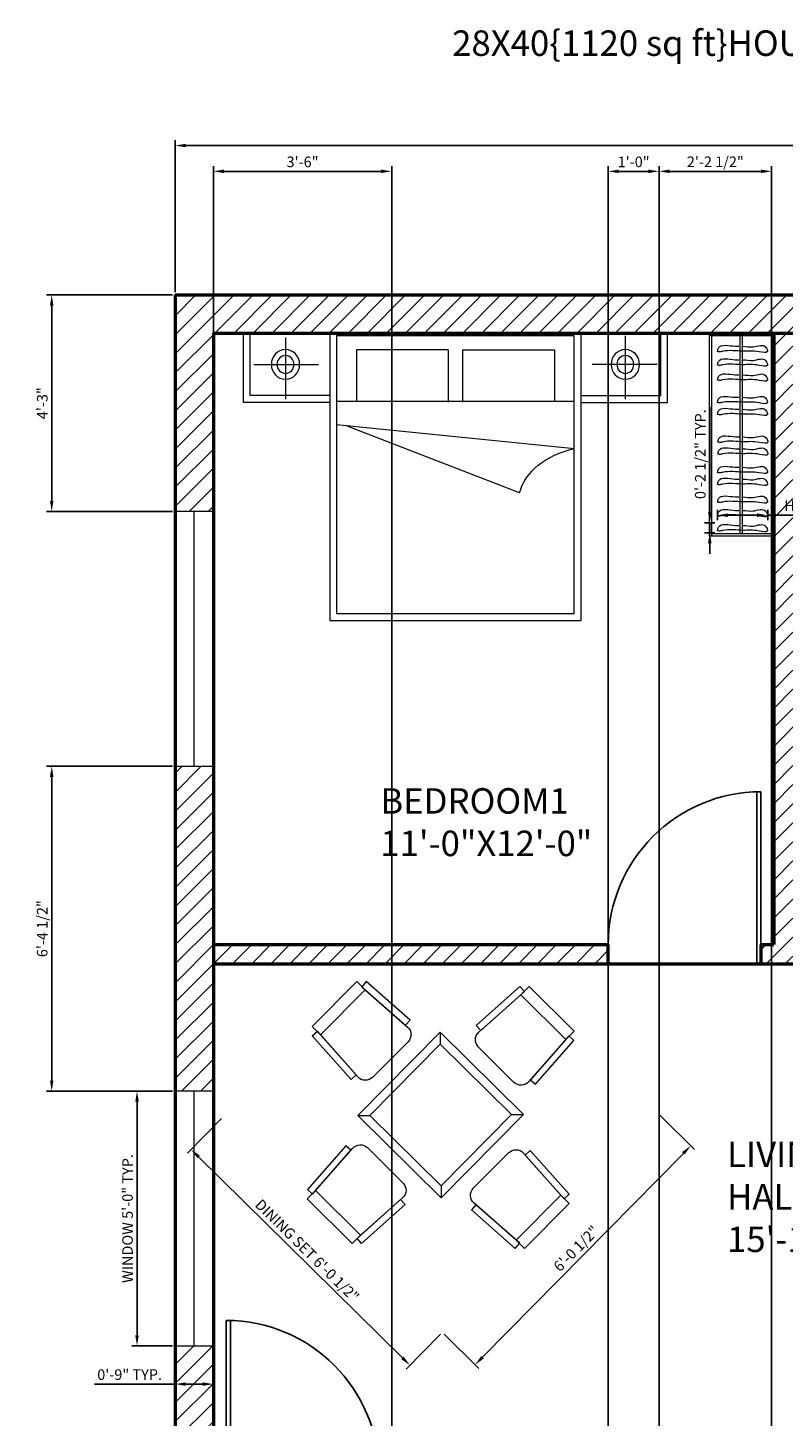
# Model space of a CAD drawing. Units: inches. Extents: x 3887 to 4286, y 884 to 1458.
# Tile 3 of 4: x 3887 to 4065, y 1131 to 1458. Entities that reach past the tile are written whole.
import ezdxf

# ---------------------------------------------------------------- set-up
doc = ezdxf.new("R2010")
doc.units = ezdxf.units.IN
for name, color, linetype, lineweight in [('A-ANNO-DIMS', 2, 'Continuous', 18), ('A-ANNO-TEXT', 7, 'Continuous', 25), ('A-AREA-IDEN', 7, 'Continuous', 25), ('A-DOOR', 3, 'Continuous', 25), ('A-FURN', 8, 'Continuous', 18), ('A-GLAZ', 4, 'Continuous', 18), ('A-WALL', 7, 'Continuous', 50), ('A-WALL-PATT', 252, 'Continuous', 13)]:
    doc.layers.add(name, color=color, linetype=linetype, lineweight=lineweight)
doc.styles.get("Standard").update_dxf_attribs({"font": 'arial.ttf'})
doc.dimstyles.new('ISO-25', dxfattribs={"dimtxt": 2.5, "dimasz": 2.5, "dimexe": 1.25, "dimexo": 0.625, "dimtad": 1, "dimdec": 0, "dimlunit": 3, "dimtxsty": 'Standard', "dimcen": 2.5, "dimadec": 0, "dimazin": 0, "dimtfac": 1, "dimtdec": 0, "dimtmove": 0, "dimatfit": 3, "dimfxl": 1, "dimarcsym": 0})

# ---------------------------------------------------------------- blocks, each defined once
blk = doc.blocks.new('4 Person Square 01')
for p, q in [((618.5, 273.1), (568.5, 323.1)), ((1268.5, 323.1), (1218.5, 273.1)), ((618.5, -326.9), (568.5, -376.9)), ((1268.5, -376.9), (1218.5, -326.9))]:
    blk.add_line(p, q)
for points in [[(734, 501.7), (693.7, 504.3), (716.8, 852.8), (757.1, 850.2)], [(755.6, 821.7), (755.9, 892.5), (1135, 890.7), (1134.7, 819.9)], [(1153.2, 499.8), (1193.6, 502), (1173.7, 850.7), (1133.4, 848.5)], [(568.5, 323.1), (1268.5, 323.1), (1268.5, -376.9), (568.5, -376.9)], [(618.5, 273.1), (1218.5, 273.1), (1218.5, -326.9), (618.5, -326.9)], [(69.9, -189.9), (-0.9, -189.6), (0.9, 189.6), (71.7, 189.3)], [(391.8, 207.8), (389.6, 248.1), (40.9, 228.3), (43.1, 188)], [(1447.2, 157.6), (1449.8, 197.9), (1798.3, 174.8), (1795.7, 134.5)], [(1767.1, 136), (1837.9, 135.7), (1836.1, -243.4), (1765.4, -243.1)], [(389.9, -211.4), (387.3, -251.7), (38.8, -228.6), (41.4, -188.3)], [(1445.2, -261.6), (1447.4, -302), (1796.1, -282.1), (1793.9, -241.8)], [(683.8, -553.6), (643.5, -555.8), (663.3, -904.5), (703.6, -902.3)], [(1103, -555.6), (1143.3, -558.2), (1120.2, -906.7), (1079.9, -904.1)], [(1081.5, -875.5), (1081.2, -946.3), (702, -944.5), (702.3, -873.8)]]:
    blk.add_lwpolyline(points, close=True)
for points in [[(1154, 483.4, -0.431982), (1093.8, 420.1), (792.7, 421.5, -0.431982), (733.1, 485.4), (755.6, 821.7), (1134.7, 819.9)], [(408.2, 208.6, -0.431982), (471.5, 148.4), (470.1, -152.7, -0.431982), (406.2, -212.3), (69.9, -189.9), (71.7, 189.3)], [(1428.9, -262.4, -0.431982), (1365.5, -202.2), (1367, 98.9, -0.431982), (1430.9, 158.5), (1767.1, 136), (1765.4, -243.1)], [(683, -537.3, -0.431982), (743.2, -473.9), (1044.3, -475.4, -0.431982), (1103.9, -539.3), (1081.5, -875.5), (702.3, -873.8)]]:
    blk.add_lwpolyline(points, format="xyb", close=True)
blk = doc.blocks.new('*D10')
at = {"layer": 'A-ANNO-DIMS', "color": 0, "lineweight": -2, "transparency": 16777216}
for p, q in [((3922.18, 1395.27), (3922.18, 1431.07)), ((3924.68, 1429.82), (4252.68, 1429.82)), ((4255.18, 1395.27), (4255.18, 1431.07))]:
    blk.add_line(p, q, dxfattribs=at)
at = {"layer": 'A-ANNO-DIMS', "color": 0, "transparency": 16777216}
for points in [[(3924.68, 1430.23), (3924.68, 1429.4), (3922.18, 1429.82)], [(4252.68, 1430.23), (4252.68, 1429.4), (4255.18, 1429.82)]]:
    blk.add_solid(points, dxfattribs=at)
at = {"layer": 'Defpoints', "color": 0, "transparency": 16777216}
for p in [(4255.18, 1429.82), (3922.18, 1394.64), (4255.18, 1394.64)]:
    blk.add_point(p, dxfattribs=at)
at = {"layer": 'A-ANNO-DIMS', "color": 0, "transparency": 16777216, "insert": (4088.68, 1431.72), "char_height": 2.5, "attachment_point": 5}
blk.add_mtext('27\'-9"', dxfattribs=at)
blk = doc.blocks.new('DOOR-SWING-36IN')
for p, q in [((35, 0), (35, 40.5)), ((36, 4.5), (36, 40.5))]:
    blk.add_line(p, q)
blk.add_arc((36, 4.5), 36, 90, 180)
blk = doc.blocks.new('WIN-GLAZ-60IN')
for p, q in [((60, 9), (0, 9)), ((0, 4.5), (60, 4.5)), ((0, 0), (60, 0))]:
    blk.add_line(p, q)
blk = doc.blocks.new('CLOSET-HANGER')
for points, knots in [([(5.84, 1.53), (5.89, 1.53), (6.71, 1.5), (8.51, 1.02), (11.18, 2.34), (12.19, -0.34), (8.75, 0.58), (5.91, 0.14), (2.52, 0.71), (0.53, 0.12), (0.14, 0.25), (0, 0.3)], [256.949798, 256.949798, 256.949798, 256.949798, 263.372126, 359.428036, 478.655159, 522.640662, 597.66786, 752.004169, 941.88133, 973.527729, 990.309099, 990.309099, 990.309099, 990.309099]), ([(0.03, 0.25), (0.09, 0.56), (0.4, 2.27), (3.16, 1.49), (4.81, 1.52), (5.08, 1.53)], [0, 0, 0, 0, 35.911014, 192.421107, 225.897258, 225.897258, 225.897258, 225.897258])]:
    blk.add_open_spline(points, degree=3, knots=knots)
blk = doc.blocks.new('*D15')
at = {"layer": 'A-ANNO-DIMS', "color": 0, "lineweight": -2, "transparency": 16777216}
for p, q in [((4049.91, 1341.61), (4049.91, 1344.01)), ((4061.79, 1341.61), (4061.79, 1344.01)), ((4052.41, 1342.76), (4059.29, 1342.76)), ((4061.79, 1342.76), (4096.55, 1342.76))]:
    blk.add_line(p, q, dxfattribs=at)
at = {"layer": 'A-ANNO-DIMS', "color": 0, "transparency": 16777216}
for points in [[(4052.41, 1343.18), (4052.41, 1342.35), (4049.91, 1342.76)], [(4059.29, 1343.18), (4059.29, 1342.35), (4061.79, 1342.76)]]:
    blk.add_solid(points, dxfattribs=at)
at = {"layer": 'Defpoints', "color": 0, "transparency": 16777216}
for p in [(4049.91, 1340.98), (4061.79, 1342.76), (4061.79, 1340.98)]:
    blk.add_point(p, dxfattribs=at)
at = {"layer": 'A-ANNO-DIMS', "color": 0, "transparency": 16777216, "insert": (4080.42, 1344.68), "char_height": 2.5, "attachment_point": 5}
blk.add_mtext('HANGER 1\'-0" TYP.', dxfattribs=at)
blk = doc.blocks.new('*D16')
at = {"layer": 'A-ANNO-DIMS', "color": 0, "lineweight": -2, "transparency": 16777216}
for p, q in [((4048.13, 1343.48), (4048.13, 1368.3)), ((4049.29, 1340.98), (4046.88, 1340.98)), ((4048.13, 1338.64), (4048.13, 1340.98)), ((4049.29, 1338.64), (4046.88, 1338.64)), ((4048.13, 1336.14), (4048.13, 1333.64))]:
    blk.add_line(p, q, dxfattribs=at)
at = {"layer": 'A-ANNO-DIMS', "color": 0, "transparency": 16777216}
for points in [[(4047.71, 1343.48), (4048.55, 1343.48), (4048.13, 1340.98)], [(4047.71, 1336.14), (4048.55, 1336.14), (4048.13, 1338.64)]]:
    blk.add_solid(points, dxfattribs=at)
at = {"layer": 'Defpoints', "color": 0, "transparency": 16777216}
for p in [(4048.13, 1340.98), (4049.91, 1340.98), (4049.91, 1338.64)]:
    blk.add_point(p, dxfattribs=at)
at = {"layer": 'A-ANNO-DIMS', "color": 0, "transparency": 16777216, "insert": (4046.21, 1357.14), "char_height": 2.5, "attachment_point": 5, "rotation": 90}
blk.add_mtext('0\'-2 1/2" TYP.', dxfattribs=at)
blk = doc.blocks.new('*D17')
at = {"layer": 'A-ANNO-DIMS', "color": 0, "lineweight": -2, "transparency": 16777216}
for p, q in [((3921.56, 1207.14), (3911.93, 1207.14)), ((3913.18, 1149.64), (3913.18, 1204.64)), ((3921.56, 1147.14), (3911.93, 1147.14))]:
    blk.add_line(p, q, dxfattribs=at)
at = {"layer": 'A-ANNO-DIMS', "color": 0, "transparency": 16777216}
for points in [[(3912.77, 1204.64), (3913.6, 1204.64), (3913.18, 1207.14)], [(3912.77, 1149.64), (3913.6, 1149.64), (3913.18, 1147.14)]]:
    blk.add_solid(points, dxfattribs=at)
at = {"layer": 'Defpoints', "color": 0, "transparency": 16777216}
for p in [(3913.18, 1207.14), (3922.18, 1207.14), (3922.18, 1147.14)]:
    blk.add_point(p, dxfattribs=at)
at = {"layer": 'A-ANNO-DIMS', "color": 0, "transparency": 16777216, "insert": (3911.27, 1177.14), "char_height": 2.5, "attachment_point": 5, "rotation": 90}
blk.add_mtext('WINDOW 5\'-0" TYP.', dxfattribs=at)
blk = doc.blocks.new('*D18')
at = {"layer": 'A-ANNO-DIMS', "color": 0, "lineweight": -2, "transparency": 16777216}
for p, q in [((3922.18, 1146.52), (3922.18, 1136.89)), ((3931.18, 1146.52), (3931.18, 1136.89)), ((3922.18, 1138.14), (3903.2, 1138.14)), ((3928.68, 1138.14), (3924.68, 1138.14))]:
    blk.add_line(p, q, dxfattribs=at)
at = {"layer": 'A-ANNO-DIMS', "color": 0, "transparency": 16777216}
for points in [[(3924.68, 1138.56), (3924.68, 1137.73), (3922.18, 1138.14)], [(3928.68, 1138.56), (3928.68, 1137.73), (3931.18, 1138.14)]]:
    blk.add_solid(points, dxfattribs=at)
at = {"layer": 'Defpoints', "color": 0, "transparency": 16777216}
for p in [(3922.18, 1147.14), (3931.18, 1147.14), (3922.18, 1138.14)]:
    blk.add_point(p, dxfattribs=at)
at = {"layer": 'A-ANNO-DIMS', "color": 0, "transparency": 16777216, "insert": (3911.44, 1140.05), "char_height": 2.5, "attachment_point": 5}
blk.add_mtext('0\'-9" TYP.', dxfattribs=at)
blk = doc.blocks.new('*D25')
at = {"layer": 'A-ANNO-DIMS', "color": 0, "lineweight": -2, "transparency": 16777216}
for p, q in [((3933.1, 1200.69), (3925.04, 1192.51)), ((3975.7, 1144.34), (3927.7, 1191.65)), ((3984.66, 1149.88), (3976.6, 1141.7))]:
    blk.add_line(p, q, dxfattribs=at)
at = {"layer": 'A-ANNO-DIMS', "color": 0, "transparency": 16777216}
for points in [[(3927.99, 1191.95), (3927.41, 1191.35), (3925.92, 1193.4)], [(3975.99, 1144.64), (3975.41, 1144.05), (3977.48, 1142.59)]]:
    blk.add_solid(points, dxfattribs=at)
at = {"layer": 'Defpoints', "color": 0, "transparency": 16777216}
for p in [(3933.54, 1201.14), (3925.92, 1193.4), (3985.1, 1150.32)]:
    blk.add_point(p, dxfattribs=at)
at = {"layer": 'A-ANNO-DIMS', "color": 0, "transparency": 16777216, "insert": (3953.05, 1169.36), "char_height": 2.5, "attachment_point": 5, "rotation": 315.4193}
blk.add_mtext('DINING SET 6\'-0 1/2"', dxfattribs=at)
blk = doc.blocks.new('*D26')
at = {"layer": 'A-ANNO-DIMS', "color": 0, "lineweight": -2, "transparency": 16777216}
for p, q in [((4036.36, 1201.45), (4044.54, 1193.39)), ((4041.9, 1192.48), (3994.59, 1144.48)), ((3985.55, 1149.88), (3993.73, 1141.82))]:
    blk.add_line(p, q, dxfattribs=at)
at = {"layer": 'A-ANNO-DIMS', "color": 0, "transparency": 16777216}
for points in [[(4041.6, 1192.78), (4042.2, 1192.19), (4043.65, 1194.27)], [(3994.3, 1144.77), (3994.89, 1144.19), (3992.84, 1142.7)]]:
    blk.add_solid(points, dxfattribs=at)
at = {"layer": 'Defpoints', "color": 0, "transparency": 16777216}
for p in [(4035.92, 1201.89), (3985.1, 1150.32), (3992.84, 1142.7)]:
    blk.add_point(p, dxfattribs=at)
at = {"layer": 'A-ANNO-DIMS', "color": 0, "transparency": 16777216, "insert": (4016.88, 1169.83), "char_height": 2.5, "attachment_point": 5, "rotation": 45.4193}
blk.add_mtext('6\'-0 1/2"', dxfattribs=at)
blk = doc.blocks.new('*D31')
at = {"layer": 'A-ANNO-DIMS', "color": 0, "lineweight": -2, "transparency": 16777216}
for p, q in [((3921.56, 1394.64), (3891.83, 1394.64)), ((3893.08, 1346.14), (3893.08, 1392.14)), ((3921.56, 1343.64), (3891.83, 1343.64))]:
    blk.add_line(p, q, dxfattribs=at)
at = {"layer": 'A-ANNO-DIMS', "color": 0, "transparency": 16777216}
for points in [[(3892.67, 1392.14), (3893.5, 1392.14), (3893.08, 1394.64)], [(3892.67, 1346.14), (3893.5, 1346.14), (3893.08, 1343.64)]]:
    blk.add_solid(points, dxfattribs=at)
at = {"layer": 'Defpoints', "color": 0, "transparency": 16777216}
for p in [(3893.08, 1394.64), (3922.18, 1394.64), (3922.18, 1343.64)]:
    blk.add_point(p, dxfattribs=at)
at = {"layer": 'A-ANNO-DIMS', "color": 0, "transparency": 16777216, "insert": (3891.18, 1369.14), "char_height": 2.5, "attachment_point": 5, "rotation": 90}
blk.add_mtext('4\'-3"', dxfattribs=at)
blk = doc.blocks.new('*D32')
at = {"layer": 'A-ANNO-DIMS', "color": 0, "lineweight": -2, "transparency": 16777216}
for p, q in [((3921.56, 1283.64), (3891.83, 1283.64)), ((3893.08, 1209.64), (3893.08, 1281.14)), ((3921.56, 1207.14), (3891.83, 1207.14))]:
    blk.add_line(p, q, dxfattribs=at)
at = {"layer": 'A-ANNO-DIMS', "color": 0, "transparency": 16777216}
for points in [[(3892.67, 1281.14), (3893.5, 1281.14), (3893.08, 1283.64)], [(3892.67, 1209.64), (3893.5, 1209.64), (3893.08, 1207.14)]]:
    blk.add_solid(points, dxfattribs=at)
at = {"layer": 'Defpoints', "color": 0, "transparency": 16777216}
for p in [(3893.08, 1283.64), (3922.18, 1283.64), (3922.18, 1207.14)]:
    blk.add_point(p, dxfattribs=at)
at = {"layer": 'A-ANNO-DIMS', "color": 0, "transparency": 16777216, "insert": (3891.17, 1245.39), "char_height": 2.5, "attachment_point": 5, "rotation": 90}
blk.add_mtext('6\'-4 1/2"', dxfattribs=at)
blk = doc.blocks.new('*D45')
at = {"layer": 'A-ANNO-DIMS', "color": 0, "lineweight": -2, "transparency": 16777216}
for p, q in [((4024.18, 966.27), (4024.18, 1424.99)), ((4026.68, 1423.74), (4033.68, 1423.74)), ((4036.18, 966.27), (4036.18, 1424.99))]:
    blk.add_line(p, q, dxfattribs=at)
at = {"layer": 'A-ANNO-DIMS', "color": 0, "transparency": 16777216}
for points in [[(4026.68, 1424.16), (4026.68, 1423.33), (4024.18, 1423.74)], [(4033.68, 1424.16), (4033.68, 1423.33), (4036.18, 1423.74)]]:
    blk.add_solid(points, dxfattribs=at)
at = {"layer": 'Defpoints', "color": 0, "transparency": 16777216}
for p in [(4036.18, 1423.74), (4024.18, 965.64), (4036.18, 965.64)]:
    blk.add_point(p, dxfattribs=at)
at = {"layer": 'A-ANNO-DIMS', "color": 0, "transparency": 16777216, "insert": (4030.18, 1425.65), "char_height": 2.5, "attachment_point": 5}
blk.add_mtext('1\'-0"', dxfattribs=at)
blk = doc.blocks.new('*D46')
at = {"layer": 'A-ANNO-DIMS', "color": 0, "lineweight": -2, "transparency": 16777216}
for p, q in [((4036.18, 966.27), (4036.18, 1424.99)), ((4038.68, 1423.74), (4060.18, 1423.74)), ((4062.68, 966.27), (4062.68, 1424.99))]:
    blk.add_line(p, q, dxfattribs=at)
at = {"layer": 'A-ANNO-DIMS', "color": 0, "transparency": 16777216}
for points in [[(4038.68, 1424.16), (4038.68, 1423.33), (4036.18, 1423.74)], [(4060.18, 1424.16), (4060.18, 1423.33), (4062.68, 1423.74)]]:
    blk.add_solid(points, dxfattribs=at)
at = {"layer": 'Defpoints', "color": 0, "transparency": 16777216}
for p in [(4062.68, 1423.74), (4036.18, 965.64), (4062.68, 965.64)]:
    blk.add_point(p, dxfattribs=at)
at = {"layer": 'A-ANNO-DIMS', "color": 0, "transparency": 16777216, "insert": (4049.43, 1425.66), "char_height": 2.5, "attachment_point": 5}
blk.add_mtext('2\'-2 1/2"', dxfattribs=at)
blk = doc.blocks.new('*D52')
at = {"layer": 'A-ANNO-DIMS', "color": 0, "lineweight": -2, "transparency": 16777216}
for p, q in [((3931.18, 1056.27), (3931.18, 1424.99)), ((3933.68, 1423.74), (3970.68, 1423.74)), ((3973.18, 1056.27), (3973.18, 1424.99))]:
    blk.add_line(p, q, dxfattribs=at)
at = {"layer": 'A-ANNO-DIMS', "color": 0, "transparency": 16777216}
for points in [[(3933.68, 1424.16), (3933.68, 1423.33), (3931.18, 1423.74)], [(3970.68, 1424.16), (3970.68, 1423.33), (3973.18, 1423.74)]]:
    blk.add_solid(points, dxfattribs=at)
at = {"layer": 'Defpoints', "color": 0, "transparency": 16777216}
for p in [(3973.18, 1423.74), (3931.18, 1055.64), (3973.18, 1055.64)]:
    blk.add_point(p, dxfattribs=at)
at = {"layer": 'A-ANNO-DIMS', "color": 0, "transparency": 16777216, "insert": (3952.18, 1425.65), "char_height": 2.5, "attachment_point": 5}
blk.add_mtext('3\'-6"', dxfattribs=at)

msp = doc.modelspace()

# ---------------------------------------------------------------- hatches: boundary and pattern name
at = {"layer": 'A-WALL-PATT'}
h = msp.add_hatch(dxfattribs=at)
h.set_pattern_fill('ANSI31', color=256)
h.paths.add_polyline_path([(4079.68, 1394.64), (3922.18, 1394.64), (3922.18, 1343.64), (3931.18, 1343.64), (3931.18, 1385.64), (4079.68, 1385.64)])
h.paths.add_polyline_path([(4156.18, 1394.64), (4109.68, 1394.64), (4109.68, 1385.64), (4156.18, 1385.64)])
h.paths.add_polyline_path([(4255.18, 1394.64), (4216.18, 1394.64), (4216.18, 1385.64), (4246.18, 1385.64), (4246.18, 1343.64), (4255.18, 1343.64)])
h.paths.add_polyline_path([(3931.18, 1283.64), (3922.18, 1283.64), (3922.18, 1207.14), (3931.18, 1207.14)])
h.paths.add_polyline_path([(4024.18, 1241.64), (3931.18, 1241.64), (3931.18, 1237.14), (4024.18, 1237.14)])
h.paths.add_polyline_path([(4067.68, 1291.14), (4079.68, 1291.14), (4079.68, 1295.64), (4067.68, 1295.64), (4067.68, 1385.64), (4063.18, 1385.64), (4063.18, 1241.64), (4060.18, 1241.64), (4060.18, 1237.14), (4067.68, 1237.14)])
h.paths.add_polyline_path([(4126.18, 1385.64), (4121.68, 1385.64), (4121.68, 1295.64), (4109.68, 1295.64), (4109.68, 1291.14), (4121.68, 1291.14), (4121.68, 1280.64), (4126.18, 1280.64)])
h.paths.add_polyline_path([(4246.18, 1241.64), (4126.18, 1241.64), (4126.18, 1244.64), (4121.68, 1244.64), (4121.68, 1156.14), (4126.18, 1156.14), (4126.18, 1237.14), (4246.18, 1237.14)])
h.paths.add_polyline_path([(4255.18, 1283.64), (4246.18, 1283.64), (4246.18, 1210.14), (4255.18, 1210.14)])
h.paths.add_polyline_path([(4255.18, 1150.14), (4246.18, 1150.14), (4246.18, 1073.64), (4255.18, 1073.64)])
h.paths.add_polyline_path([(4246.18, 1117.14), (4126.18, 1117.14), (4126.18, 1120.14), (4121.68, 1120.14), (4121.68, 1117.14), (4119.68, 1117.14), (4119.68, 1112.64), (4246.18, 1112.64)])
h.paths.add_polyline_path([(4079.18, 1112.64), (4083.68, 1112.64), (4083.68, 1117.14), (4074.68, 1117.14), (4074.68, 974.64), (4079.18, 974.64)])
h.paths.add_polyline_path([(4019.68, 1117.14), (3970.18, 1117.14), (3970.18, 1112.64), (4015.18, 1112.64), (4015.18, 974.64), (4019.68, 974.64), (4019.68, 1058.64), (4021.68, 1058.64), (4021.68, 1063.14), (4019.68, 1063.14)])
h.paths.add_polyline_path([(3931.18, 1147.14), (3922.18, 1147.14), (3922.18, 917.64), (3933.18, 917.64), (3933.18, 926.64), (3931.18, 926.64)])
h.paths.add_polyline_path([(4024.18, 965.64), (4036.18, 965.64), (4036.18, 974.64), (4015.18, 974.64), (4015.18, 926.64), (4003.18, 926.64), (4003.18, 917.64), (4024.18, 917.64)])
h.paths.add_polyline_path([(4132.68, 974.64), (4062.68, 974.64), (4062.68, 965.64), (4132.68, 965.64)])
h.paths.add_polyline_path([(4255.18, 1013.64), (4246.18, 1013.64), (4246.18, 974.64), (4192.68, 974.64), (4192.68, 965.64), (4255.18, 965.64)])

# ---------------------------------------------------------------- linework, layer by layer
at = {"layer": 'A-FURN'}
for p, q in [((3938.27, 1385.64), (4038.16, 1385.64)), ((3938.27, 1369.3), (3938.27, 1385.64)), ((3939.83, 1370.93), (3939.83, 1385.64)), ((3948.16, 1384.62), (3948.16, 1370.09)), ((3958.63, 1385.64), (3958.63, 1317.96)), ((4016.21, 1384.99), (3960.19, 1384.99)), ((3960.19, 1384.99), (3960.19, 1319.59)), ((4016.21, 1319.59), (4016.21, 1384.99)), ((4017.8, 1317.96), (4017.8, 1385.64)), ((4028.23, 1384.98), (4028.23, 1370.09)), ((4036.6, 1370.93), (4036.6, 1385.64)), ((4038.16, 1369.3), (4038.16, 1385.64)), ((4048, 1385.61), (4048, 1337.92)), ((4048, 1385.61), (4063.16, 1385.61)), ((4048, 1385.1), (4063.16, 1385.1)), ((4048.51, 1385.61), (4048.51, 1337.92)), ((4055.22, 1385.61), (4055.22, 1338.43)), ((4055.73, 1385.61), (4055.73, 1338.43)), ((4062.65, 1337.92), (4062.65, 1385.61)), ((4063.16, 1337.92), (4063.16, 1385.61)), ((3986.51, 1381.72), (3964.86, 1381.72)), ((3964.86, 1381.72), (3964.86, 1369.51)), ((3986.51, 1381.72), (3986.51, 1369.4)), ((3989.88, 1381.72), (4011.54, 1381.72)), ((3989.88, 1381.72), (3989.88, 1369.4)), ((4011.54, 1381.72), (4011.54, 1369.51)), ((3940.69, 1378.27), (3955.95, 1378.27)), ((4035.7, 1378.27), (4020.45, 1378.27)), ((3958.52, 1370.93), (3939.83, 1370.93)), ((4017.92, 1370.93), (4036.6, 1370.93)), ((3958.52, 1369.3), (3938.27, 1369.3)), ((4016.19, 1369.51), (3960.18, 1369.51)), ((4017.92, 1369.3), (4038.16, 1369.3)), ((3960.21, 1364.12), (4016.24, 1358.45)), ((4003.33, 1348.02), (3962.33, 1363.92)), ((4048, 1338.43), (4063.16, 1338.43)), ((4048, 1337.92), (4063.16, 1337.92)), ((3958.63, 1317.96), (4017.8, 1317.96)), ((3960.19, 1319.59), (4016.21, 1319.59))]:
    msp.add_line(p, q, dxfattribs=at)
at = {"layer": 'A-FURN', "extrusion": (0, 0, -1)}
for centre in [(3948.16, 1378.27), (4028.23, 1378.27)]:
    msp.add_ellipse(centre, major_axis=(0, -3.5), ratio=0.952381, dxfattribs=at)
for centre, major_axis, ratio, start_param, end_param in [((3948.16, 1378.27), (0, -2.1), 0.952381, 3.141593, 9.424778), ((4028.23, 1378.27), (0, -2.1), 0.952381, 3.141593, 9.424778), ((4021.94, 1345.86), (18.86, 0), 0.700439, 3.305513, 4.405354)]:
    msp.add_ellipse(centre, major_axis=major_axis, ratio=ratio, start_param=start_param, end_param=end_param, dxfattribs=at)
at = {"layer": 'A-GLAZ'}
for p, q in [((3931.18, 1343.64), (3922.18, 1343.64)), ((3922.18, 1283.64), (3931.18, 1283.64)), ((3931.18, 1207.14), (3922.18, 1207.14)), ((3922.18, 1147.14), (3931.18, 1147.14))]:
    msp.add_line(p, q, dxfattribs=at)
at = {"layer": 'A-WALL'}
for p, q in [((3922.18, 1394.64), (4255.18, 1394.64)), ((3922.18, 1394.64), (3922.18, 917.64)), ((3931.18, 1385.64), (4246.18, 1385.64)), ((3931.18, 1385.64), (3931.18, 926.64)), ((4063.18, 1385.64), (4063.18, 1241.64)), ((3931.18, 1241.64), (4024.18, 1241.64)), ((4024.18, 1237.14), (4024.18, 1241.64)), ((4060.18, 1241.64), (4060.18, 1237.14)), ((4060.18, 1241.64), (4063.18, 1241.64)), ((3931.18, 1237.14), (4067.68, 1237.14))]:
    msp.add_line(p, q, dxfattribs=at)

# ---------------------------------------------------------------- block references
at = {"layer": 'A-DOOR'}
msp.add_blockref('DOOR-SWING-36IN', (4024.18, 1237.14), dxfattribs=at)
at = {"layer": 'A-DOOR', "extrusion": (0, 0, -1), "zscale": -1}
msp.add_blockref('DOOR-SWING-36IN', (-3970.18, 1112.64), dxfattribs=at)
at = {"layer": 'A-FURN'}
for p in [(4049.91, 1381.04), (4049.91, 1377.85), (4049.91, 1374.31), (4049.91, 1369.02), (4049.91, 1366.21), (4049.99, 1359.7), (4049.99, 1356.89), (4049.91, 1352.55), (4049.91, 1349.75), (4049.91, 1345.56), (4049.91, 1342.38), (4049.91, 1338.84)]:
    msp.add_blockref('CLOSET-HANGER', p, dxfattribs=at)
at = {"layer": 'A-FURN', "xscale": 0.0393700787401575, "yscale": 0.0393700787401575, "zscale": 0.0393700787401575, "rotation": 135.4192636555872}
msp.add_blockref('4 Person Square 01', (4009.74, 1175.38), dxfattribs=at)
at = {"layer": 'A-GLAZ', "rotation": 90.00000000000104}
for p in [(3931.18, 1283.64), (3931.18, 1147.14)]:
    msp.add_blockref('WIN-GLAZ-60IN', p, dxfattribs=at)

# ---------------------------------------------------------------- texts
at = {"layer": 'A-ANNO-TEXT', "insert": (3987.44, 1456.93), "char_height": 6, "attachment_point": 1}
msp.add_mtext_dynamic_manual_height_columns('28X40\\{1120 sq ft\\}HOUSE PLAN-WEST FACE-FP1316', width=229.9608, gutter_width=12.5, heights=[8.06], dxfattribs=at)
at = {"layer": 'A-AREA-IDEN', "insert": (3970.51, 1278.48), "char_height": 6, "attachment_point": 1}
msp.add_mtext('BEDROOM1\\P11\'-0"X12\'-0"', dxfattribs=at)
at = {"layer": 'A-AREA-IDEN', "insert": (4052.2, 1195.24), "char_height": 6, "attachment_point": 1}
msp.add_mtext_dynamic_manual_height_columns('LIVING HALL\\P15\'-11"X10\'-0"', width=9.7433, gutter_width=12.5, heights=[0], dxfattribs=at)

# ---------------------------------------------------------------- dimensions: what is measured, and where the dimension line sits
at = {"layer": 'A-ANNO-DIMS'}
for base, p1, p2, override, picture, middle in [((4255.18, 1429.82), (3922.18, 1394.64), (4255.18, 1394.64), {"dimclrd": 0, "dimclre": 0, "dimclrt": 0}, '*D10', (4088.68, 1431.72)), ((4062.68, 1423.74), (4036.18, 965.64), (4062.68, 965.64), {"dimdec": 1, "dimlfac": 1, "dimrnd": 0, "dimzin": 1, "dimdsep": 46, "dimlunit": 4, "dimfrac": 2}, '*D46', (4049.43, 1425.66)), ((3973.18, 1423.74), (3931.18, 1055.64), (3973.18, 1055.64), {"dimdec": 1, "dimlfac": 1, "dimrnd": 0, "dimzin": 1, "dimdsep": 46, "dimlunit": 4, "dimfrac": 2}, '*D52', (3952.18, 1425.65)), ((4036.18, 1423.74), (4024.18, 965.64), (4036.18, 965.64), {"dimdec": 1, "dimlfac": 1, "dimrnd": 0, "dimzin": 1, "dimdsep": 46, "dimlunit": 4, "dimfrac": 2}, '*D45', (4030.18, 1425.65))]:
    dim = msp.add_linear_dim(base=base, p1=p1, p2=p2, dimstyle='ISO-25', override=override, dxfattribs=at)
    dim.commit()
    dim.dimension.update_dxf_attribs({"geometry": picture, "text_midpoint": middle})
for base, p1, p2, angle, picture, middle in [((3893.08, 1394.64), (3922.18, 1343.64), (3922.18, 1394.64), 90, '*D31', (3891.18, 1369.14)), ((3893.08, 1283.64), (3922.18, 1207.14), (3922.18, 1283.64), 90, '*D32', (3891.17, 1245.39)), ((3992.84, 1142.7), (4035.92, 1201.89), (3985.1, 1150.32), 225.4193, '*D26', (4016.88, 1169.83))]:
    dim = msp.add_linear_dim(base=base, p1=p1, p2=p2, angle=angle, dimstyle='ISO-25', override={"dimdec": 1, "dimlfac": 1, "dimrnd": 0, "dimzin": 1, "dimdsep": 46, "dimlunit": 4, "dimfrac": 2}, dxfattribs=at)
    dim.commit()
    dim.dimension.update_dxf_attribs({"geometry": picture, "text_midpoint": middle})
for base, p1, p2, angle, text, picture, middle in [((4048.13, 1340.98), (4049.91, 1338.64), (4049.91, 1340.98), 90, '<> TYP.', '*D16', (4046.21, 1357.14)), ((3913.18, 1207.14), (3922.18, 1147.14), (3922.18, 1207.14), 90, 'WINDOW <> TYP.', '*D17', (3911.27, 1177.14)), ((3925.92, 1193.4), (3985.1, 1150.32), (3933.54, 1201.14), 135.4193, 'DINING SET <>', '*D25', (3953.05, 1169.36)), ((3922.18, 1138.14), (3931.18, 1147.14), (3922.18, 1147.14), 180, '<> TYP.', '*D18', (3911.44, 1140.05))]:
    dim = msp.add_linear_dim(base=base, p1=p1, p2=p2, angle=angle, text=text, dimstyle='ISO-25', override={"dimdec": 1, "dimlfac": 1, "dimrnd": 0, "dimzin": 1, "dimdsep": 46, "dimlunit": 4, "dimfrac": 2}, dxfattribs=at)
    dim.commit()
    dim.dimension.update_dxf_attribs({"geometry": picture, "text_midpoint": middle})
dim = msp.add_linear_dim(base=(4061.79, 1342.76), p1=(4049.91, 1340.98), p2=(4061.79, 1340.98), text='HANGER <> TYP.', dimstyle='ISO-25', override={"dimdec": 1, "dimlfac": 1, "dimrnd": 0, "dimzin": 1, "dimdsep": 46, "dimlunit": 4, "dimfrac": 2}, dxfattribs=at)
dim.commit()
dim.dimension.update_dxf_attribs({"geometry": '*D15', "text_midpoint": (4080.42, 1344.68)})

doc.saveas('drawing.dxf')
